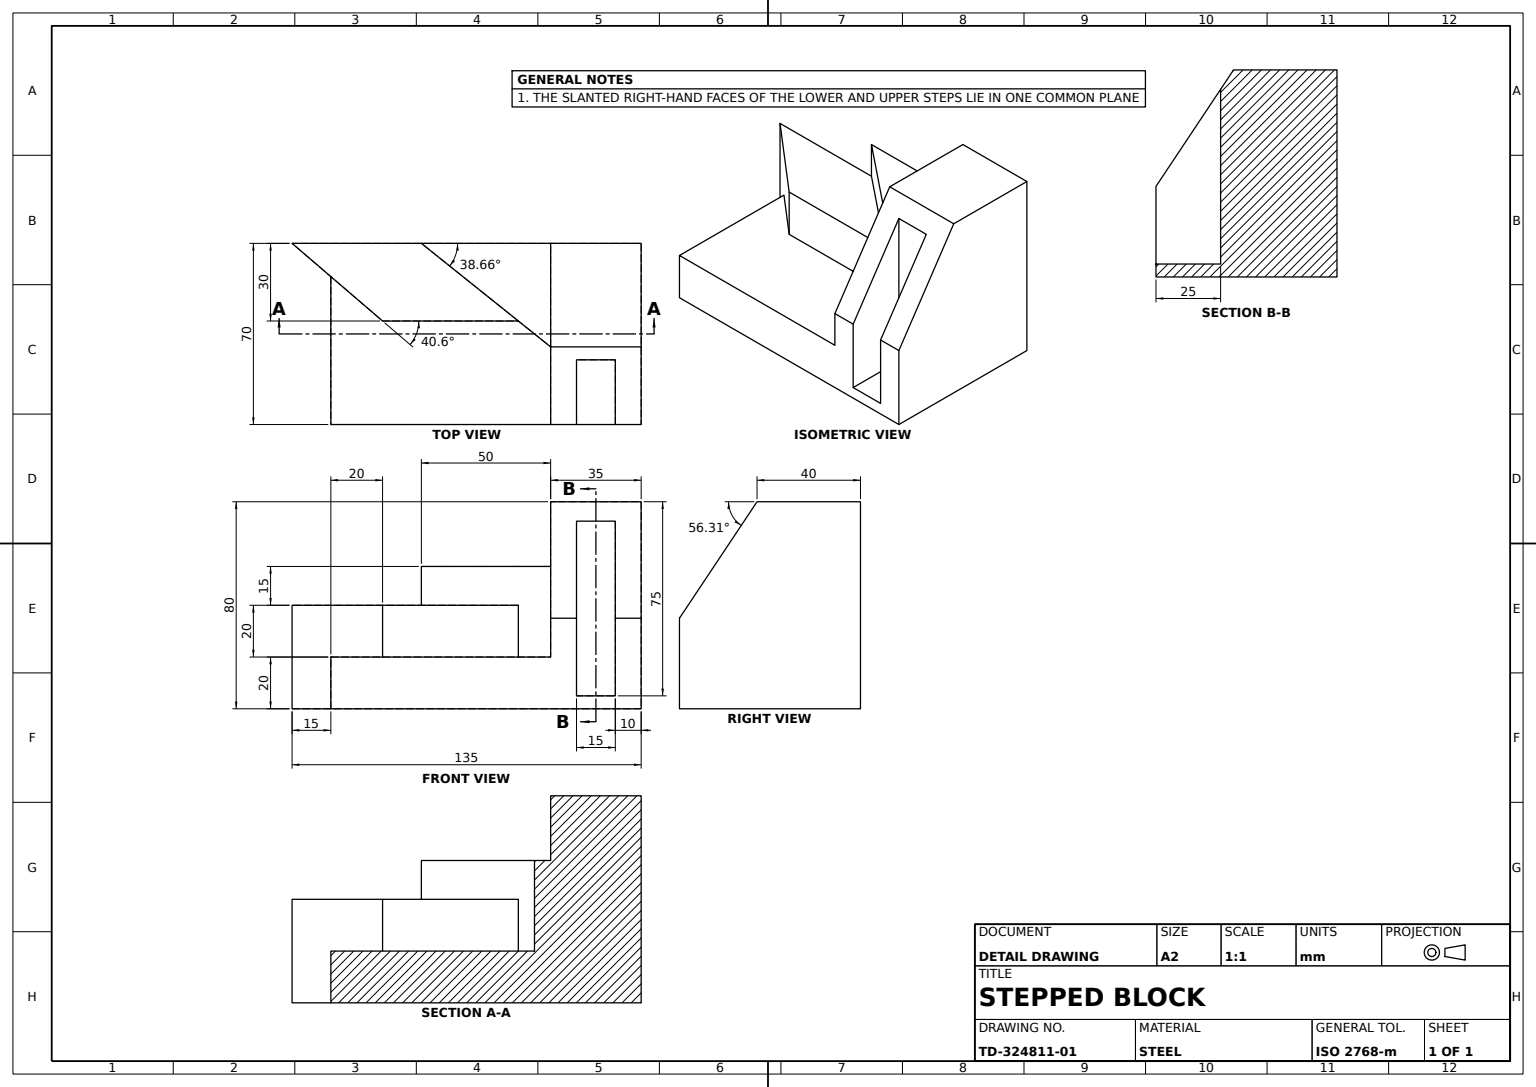
from build123d import *

# Parameters (mm, degrees)
BASE_PLATE_SKETCH_W   = 70
BASE_PLATE_SKETCH_H   = 135
BASE_PLATE_DEPTH      = 20
TOWER_DEPTH           = 35
TOWER_WINDOW_SKETCH_W = 25
TOWER_WINDOW_SKETCH_H = 15
TOWER_WINDOW_DEPTH    = 75
UPPER_STEP_DEPTH      = 35
LOWER_STEP_DEPTH      = 20
STEP_NOTCH_DEPTH      = 20


with BuildPart() as part:
    # Base Plate Sketch → Base Plate (new body)
    with BuildSketch(Plane(origin=(0, 0, 0), x_dir=(1, 0, 0), z_dir=(0, 1, 0))):
        Rectangle(BASE_PLATE_SKETCH_W, BASE_PLATE_SKETCH_H)
    extrude(amount=BASE_PLATE_DEPTH)

    # Tower Profile Sketch → Tower (add)
    with BuildSketch(Plane(origin=(0, 0, -67.5), x_dir=(-1, 0, 0), z_dir=(0, 0, -1))):
        Polygon((35, 0), (35, 80), (-5, 80), (-35, 35), (-35, 0), align=None)
    extrude(amount=-TOWER_DEPTH)

    # Tower Window Sketch → Tower Window (cut)
    with BuildSketch(Plane(origin=(0, 80, 0), x_dir=(1, 0, 0), z_dir=(0, 1, 0))):
        with Locations((22.5, 50)):
            Rectangle(TOWER_WINDOW_SKETCH_W, TOWER_WINDOW_SKETCH_H)
    extrude(amount=-TOWER_WINDOW_DEPTH, mode=Mode.SUBTRACT)

    # Upper Step Sketch → Upper Step (add)
    with BuildSketch(Plane(origin=(0, 20, 0), x_dir=(1, 0, 0), z_dir=(0, 1, 0))):
        Polygon((-35, 32.5), (5, 32.5), (-35, -17.5), align=None)
    extrude(amount=UPPER_STEP_DEPTH)

    # Lower Step Sketch → Lower Step (add)
    with BuildSketch(Plane(origin=(0, 20, 0), x_dir=(1, 0, 0), z_dir=(0, 1, 0))):
        Polygon((-35, -17.5), (-35, -67.5), (-5, -32.5), (-5, 20), align=None)
    extrude(amount=LOWER_STEP_DEPTH)

    # Step Notch Sketch → Step Notch (cut)
    with BuildSketch(Plane(origin=(0, 20, 0), x_dir=(1, 0, 0), z_dir=(0, 1, 0))):
        Polygon((35, -67.5), (35, -52.5), (-22.142857143, -52.5), (-35, -67.5), align=None)
    extrude(amount=-STEP_NOTCH_DEPTH, mode=Mode.SUBTRACT)


solid = part.part
